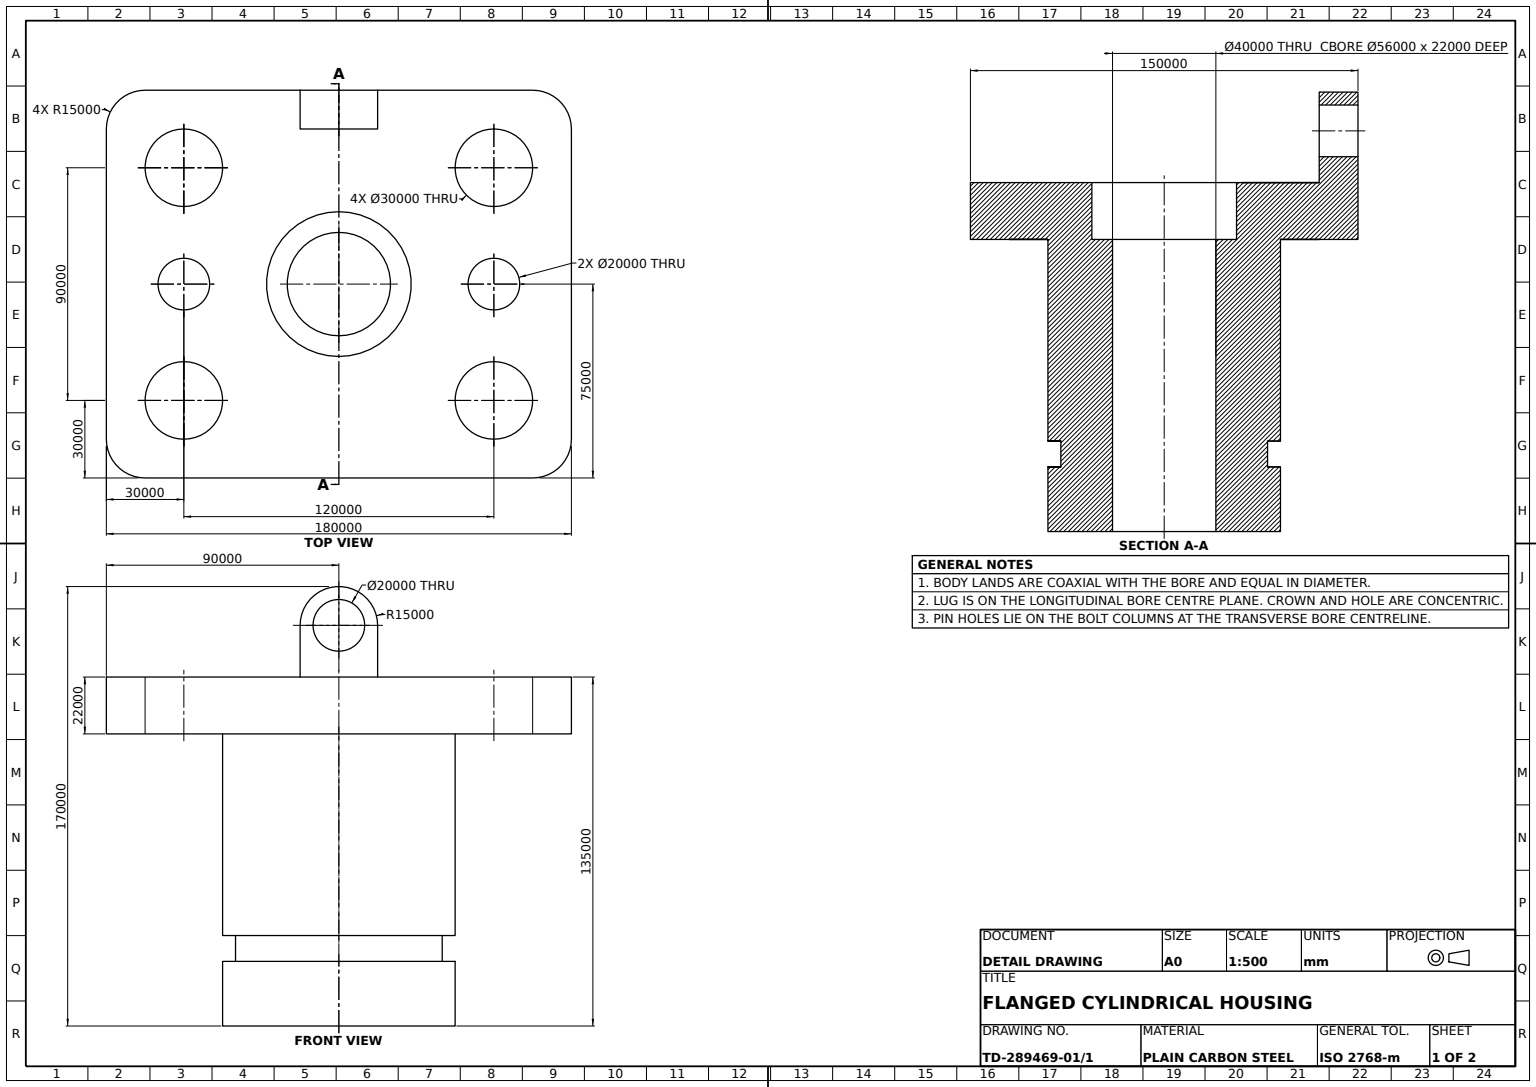
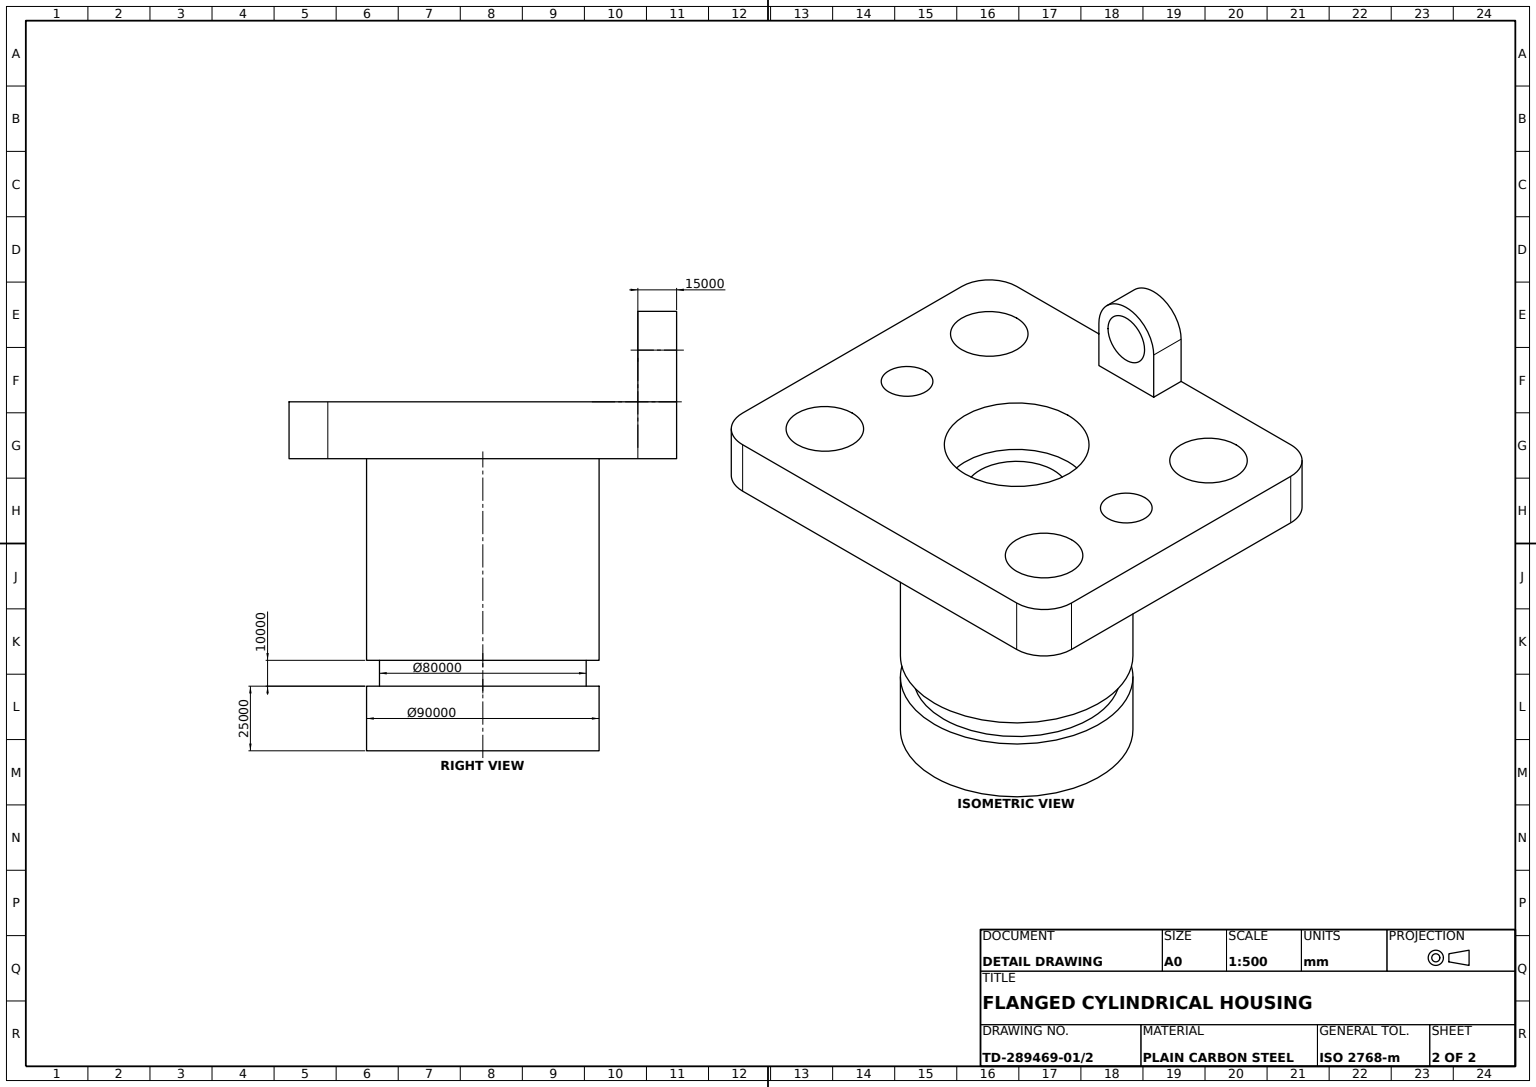
from build123d import *

# Parameters (mm, degrees)
FLANGE_PROFILE_180X150_W         = 180000
FLANGE_PROFILE_180X150_H         = 150000
SQUARE_FLANGE_DEPTH              = 22000
CENTRE_RECESS_SKETCH_R           = 28000
CENTRE_RECESS_DEPTH              = 22000
FLANGE_CORNER_FILLET_R15_A_R     = 15000
FLANGE_CORNER_FILLET_R15_B_R     = 15000
FLANGE_CORNER_FILLET_R15_C_R     = 15000
FLANGE_CORNER_FILLET_R15_D_R     = 15000
BOLT_HOLE_30_A_SKETCH_R          = 15000
BOLT_HOLE_30_A_DEPTH             = 22000
PIN_HOLE_20_A_SKETCH_R           = 10000
PIN_HOLE_20_A_DEPTH              = 22000
BOLT_HOLE_30_B_SKETCH_R          = 15000
BOLT_HOLE_30_B_DEPTH             = 22000
BOLT_HOLE_30_C_REACH             = 178747.629
BOLT_HOLE_30_C_SKETCH_R          = 15000
BOLT_HOLE_30_C_DIRECTION_2_DEPTH = 178746.629317195
PIN_HOLE_20_B_REACH              = 178747.629
PIN_HOLE_20_B_SKETCH_R           = 10000
BOLT_HOLE_30_D_REACH             = 178747.629
BOLT_HOLE_30_D_SKETCH_R          = 15000
LIFTING_LUG_DEPTH                = 15000
LIFTING_EYE_HOLE_REACH           = 243928.218
LIFTING_EYE_HOLE_SKETCH_R        = 10000


with BuildPart() as part:
    # Plug Body Profile → Plug Body (revolve)
    with BuildSketch(Plane.XY, mode=Mode.PRIVATE) as plug_body_sk:
        Polygon((-20000, 0), (-20000, 121000), (-28000, 121000), (-28000, 135000), (-53000, 135000), (-53000, 115000), (-45000, 115000), (-45000, 35000), (-40000, 35000), (-40000, 25000), (-45000, 25000), (-45000, 0), align=None)
    revolve(plug_body_sk.sketch.rotate(Axis((0, 0, 0), (0, 1, 0)), 270), axis=Axis((0, 0, 0), (0, 1, 0)))

    # Flange Profile 180x150 → Square Flange (add)
    with BuildSketch(Plane(origin=(0, 135000, 0), x_dir=(1, 0, 0), z_dir=(0, 1, 0))):
        Rectangle(FLANGE_PROFILE_180X150_W, FLANGE_PROFILE_180X150_H)
    extrude(amount=-SQUARE_FLANGE_DEPTH)

    # Centre Recess Sketch → Centre Recess (cut)
    with BuildSketch(Plane(origin=(0, 135000, 0), x_dir=(1, 0, 0), z_dir=(0, 1, 0))):
        with Locations(Location((0, 0, 0), (0, 0, 270))):
            Circle(CENTRE_RECESS_SKETCH_R)
    extrude(amount=-CENTRE_RECESS_DEPTH, mode=Mode.SUBTRACT)

    # Flange Corner Fillet R15 A
    flange_corner_fillet_r15_a_edges = [part.edges().sort_by_distance(p)[0] for p in [
        (90000, 124000, 75000),
    ]]
    fillet(flange_corner_fillet_r15_a_edges, radius=FLANGE_CORNER_FILLET_R15_A_R)

    # Flange Corner Fillet R15 B
    flange_corner_fillet_r15_b_edges = [part.edges().sort_by_distance(p)[0] for p in [
        (-90000, 124000, 75000),
    ]]
    fillet(flange_corner_fillet_r15_b_edges, radius=FLANGE_CORNER_FILLET_R15_B_R)

    # Flange Corner Fillet R15 C
    flange_corner_fillet_r15_c_edges = [part.edges().sort_by_distance(p)[0] for p in [
        (-90000, 124000, -75000),
    ]]
    fillet(flange_corner_fillet_r15_c_edges, radius=FLANGE_CORNER_FILLET_R15_C_R)

    # Flange Corner Fillet R15 D
    flange_corner_fillet_r15_d_edges = [part.edges().sort_by_distance(p)[0] for p in [
        (90000, 124000, -75000),
    ]]
    fillet(flange_corner_fillet_r15_d_edges, radius=FLANGE_CORNER_FILLET_R15_D_R)

    # Bolt Hole Ø30 A Sketch → Bolt Hole Ø30 A (cut)
    with BuildSketch(Plane(origin=(0, 135000, 0), x_dir=(1, 0, 0), z_dir=(0, 1, 0))):
        with Locations(Location((-60000, -45000, 0), (0, 0, 270))):
            Circle(BOLT_HOLE_30_A_SKETCH_R)
    extrude(amount=-BOLT_HOLE_30_A_DEPTH, mode=Mode.SUBTRACT)

    # Pin Hole Ø20 A Sketch → Pin Hole Ø20 A (cut)
    with BuildSketch(Plane(origin=(0, 135000, 0), x_dir=(1, 0, 0), z_dir=(0, 1, 0))):
        with Locations(Location((-60000, 0, 0), (0, 0, 270))):
            Circle(PIN_HOLE_20_A_SKETCH_R)
    extrude(amount=-PIN_HOLE_20_A_DEPTH, mode=Mode.SUBTRACT)

    # Bolt Hole Ø30 B Sketch → Bolt Hole Ø30 B (cut)
    with BuildSketch(Plane(origin=(0, 135000, 0), x_dir=(1, 0, 0), z_dir=(0, 1, 0))):
        with Locations(Location((-60000, 45000, 0), (0, 0, 270))):
            Circle(BOLT_HOLE_30_B_SKETCH_R)
    extrude(amount=-BOLT_HOLE_30_B_DEPTH, mode=Mode.SUBTRACT)

    # Bolt Hole Ø30 C Sketch → Bolt Hole Ø30 C (cut, up to next)
    with BuildSketch(Plane(origin=(0, 135000, 0), x_dir=(1, 0, 0), z_dir=(0, 1, 0)), mode=Mode.PRIVATE) as bolt_hole_30_c_sk1:
        with Locations(Location((60000, 45000, 0), (0, 0, 90))):
            Circle(BOLT_HOLE_30_C_SKETCH_R)
    bolt_hole_30_c_tool1 = extrude(bolt_hole_30_c_sk1.sketch, amount=-BOLT_HOLE_30_C_REACH, mode=Mode.PRIVATE) & part.part
    add(bolt_hole_30_c_tool1.solids().sort_by_distance((60000, 135000, -45000))[0], mode=Mode.SUBTRACT)

    # Bolt Hole Ø30 C Sketch → Bolt Hole Ø30 C direction 2 (cut)
    with BuildSketch(Plane(origin=(0, 135000, 0), x_dir=(1, 0, 0), z_dir=(0, 1, 0))):
        with Locations(Location((60000, 45000, 0), (0, 0, 90))):
            Circle(BOLT_HOLE_30_C_SKETCH_R)
    extrude(amount=BOLT_HOLE_30_C_DIRECTION_2_DEPTH, mode=Mode.SUBTRACT)

    # Pin Hole Ø20 B Sketch → Pin Hole Ø20 B (cut, up to next)
    with BuildSketch(Plane(origin=(0, 135000, 0), x_dir=(1, 0, 0), z_dir=(0, 1, 0)), mode=Mode.PRIVATE) as pin_hole_20_b_sk1:
        with Locations(Location((60000, 0, 0), (0, 0, 270))):
            Circle(PIN_HOLE_20_B_SKETCH_R)
    pin_hole_20_b_tool1 = extrude(pin_hole_20_b_sk1.sketch, amount=-PIN_HOLE_20_B_REACH, mode=Mode.PRIVATE) & part.part
    add(pin_hole_20_b_tool1.solids().sort_by_distance((60000, 135000, 0))[0], mode=Mode.SUBTRACT)

    # Bolt Hole Ø30 D Sketch → Bolt Hole Ø30 D (cut, up to next)
    with BuildSketch(Plane(origin=(0, 135000, 0), x_dir=(1, 0, 0), z_dir=(0, 1, 0)), mode=Mode.PRIVATE) as bolt_hole_30_d_sk1:
        with Locations(Location((60000, -45000, 0), (0, 0, 270))):
            Circle(BOLT_HOLE_30_D_SKETCH_R)
    bolt_hole_30_d_tool1 = extrude(bolt_hole_30_d_sk1.sketch, amount=-BOLT_HOLE_30_D_REACH, mode=Mode.PRIVATE) & part.part
    add(bolt_hole_30_d_tool1.solids().sort_by_distance((60000, 135000, 45000))[0], mode=Mode.SUBTRACT)

    # Lifting Lug Profile → Lifting Lug (add)
    with BuildSketch(Plane(origin=(0, 0, -75000), x_dir=(-1, 0, 0), z_dir=(0, 0, -1))):
        with BuildLine():
            Line((0, 135000), (15000, 135000))
            Line((15000, 135000), (15000, 155000))
            ThreePointArc((15000, 155000), (0, 170000), (-15000, 155000))
            Line((-15000, 155000), (-15000, 135000))
            Line((-15000, 135000), (0, 135000))
        make_face()
    extrude(amount=-LIFTING_LUG_DEPTH)

    # Lifting Eye Hole Sketch → Lifting Eye Hole (cut, up to next)
    with BuildSketch(Plane(origin=(0, 0, -75000), x_dir=(-1, 0, 0), z_dir=(0, 0, -1)), mode=Mode.PRIVATE) as lifting_eye_hole_sk1:
        with Locations((0, 155000)):
            Circle(LIFTING_EYE_HOLE_SKETCH_R)
    lifting_eye_hole_tool1 = extrude(lifting_eye_hole_sk1.sketch, amount=-LIFTING_EYE_HOLE_REACH, mode=Mode.PRIVATE) & part.part
    add(lifting_eye_hole_tool1.solids().sort_by_distance((0, 155000, -75000))[0], mode=Mode.SUBTRACT)


solid = part.part
